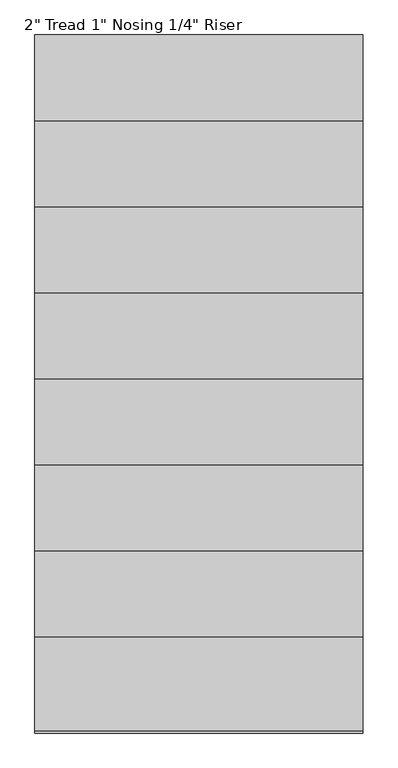
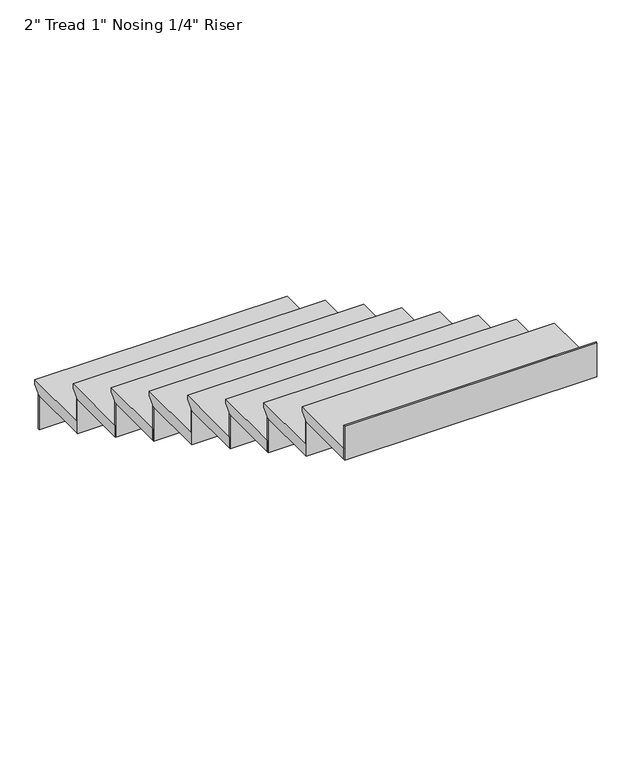
"""IFC4 building model written with IfcOpenShell, lengths in millimetres: stair flight geometry."""

from ifc_helpers import new_model, si_unit, frame, origin, place, context, project, spatial, polyline, outline, extrude, source, transform, mapped, element, save


def stair_flight_8fbc4922(model_context):
    return source(origin(), model_context, "Body", "SweptSolid", [
        extrude(outline(polyline([(-2204.7834702, 4876.8), (-1899.9834702, 4876.8), (-1899.9834702, 4857.75), (-1925.3834702, 4832.35), (-1925.3834702, 4826.0), (-2204.7834702, 4826.0), (-2204.7834702, 4876.8)])), frame((2385.53354, 0.0, 0.0), z_axis=(1.0, 0.0, 0.0), x_axis=(0.0, 1.0, 0.0)), (0.0, 0.0, 1.0), 1066.8),
        extrude(outline(polyline([(2385.53354, -1931.7334702), (2385.53354, -1925.3834702), (3452.33354, -1925.3834702), (3452.33354, -1931.7334702), (2385.53354, -1931.7334702)])), frame((0.0, 0.0, 4673.6), z_axis=(0.0, 0.0, 1.0), x_axis=(1.0, 0.0, 0.0)), (0.0, 0.0, 1.0), 152.4),
        extrude(outline(polyline([(2385.53354, -2211.1334702), (2385.53354, -2204.7834702), (3452.33354, -2204.7834702), (3452.33354, -2211.1334702), (2385.53354, -2211.1334702)])), frame((0.0, 0.0, 4826.0), z_axis=(0.0, 0.0, 1.0), x_axis=(1.0, 0.0, 0.0)), (0.0, 0.0, 1.0), 152.4),
        extrude(outline(polyline([(-2484.1834702, 5029.2), (-2179.3834702, 5029.2), (-2179.3834702, 5010.15), (-2204.7834702, 4984.75), (-2204.7834702, 4978.4), (-2484.1834702, 4978.4), (-2484.1834702, 5029.2)])), frame((2385.53354, 0.0, 0.0), z_axis=(1.0, 0.0, 0.0), x_axis=(0.0, 1.0, 0.0)), (0.0, 0.0, 1.0), 1066.8),
        extrude(outline(polyline([(2385.53354, -2490.5334702), (2385.53354, -2484.1834702), (3452.33354, -2484.1834702), (3452.33354, -2490.5334702), (2385.53354, -2490.5334702)])), frame((0.0, 0.0, 4978.4), z_axis=(0.0, 0.0, 1.0), x_axis=(1.0, 0.0, 0.0)), (0.0, 0.0, 1.0), 152.4),
        extrude(outline(polyline([(-2763.5834702, 5181.6), (-2458.7834702, 5181.6), (-2458.7834702, 5162.55), (-2484.1834702, 5137.15), (-2484.1834702, 5130.8), (-2763.5834702, 5130.8), (-2763.5834702, 5181.6)])), frame((2385.53354, 0.0, 0.0), z_axis=(1.0, 0.0, 0.0), x_axis=(0.0, 1.0, 0.0)), (0.0, 0.0, 1.0), 1066.8),
        extrude(outline(polyline([(2385.53354, -2769.9334702), (2385.53354, -2763.5834702), (3452.33354, -2763.5834702), (3452.33354, -2769.9334702), (2385.53354, -2769.9334702)])), frame((0.0, 0.0, 5130.8), z_axis=(0.0, 0.0, 1.0), x_axis=(1.0, 0.0, 0.0)), (0.0, 0.0, 1.0), 152.4),
        extrude(outline(polyline([(-3042.9834702, 5334.0), (-2738.1834702, 5334.0), (-2738.1834702, 5314.95), (-2763.5834702, 5289.55), (-2763.5834702, 5283.2), (-3042.9834702, 5283.2), (-3042.9834702, 5334.0)])), frame((2385.53354, 0.0, 0.0), z_axis=(1.0, 0.0, 0.0), x_axis=(0.0, 1.0, 0.0)), (0.0, 0.0, 1.0), 1066.8),
        extrude(outline(polyline([(2385.53354, -3049.3334702), (2385.53354, -3042.9834702), (3452.33354, -3042.9834702), (3452.33354, -3049.3334702), (2385.53354, -3049.3334702)])), frame((0.0, 0.0, 5283.2), z_axis=(0.0, 0.0, 1.0), x_axis=(1.0, 0.0, 0.0)), (0.0, 0.0, 1.0), 152.4),
        extrude(outline(polyline([(-3322.3834702, 5486.4), (-3017.5834702, 5486.4), (-3017.5834702, 5467.35), (-3042.9834702, 5441.95), (-3042.9834702, 5435.6), (-3322.3834702, 5435.6), (-3322.3834702, 5486.4)])), frame((2385.53354, 0.0, 0.0), z_axis=(1.0, 0.0, 0.0), x_axis=(0.0, 1.0, 0.0)), (0.0, 0.0, 1.0), 1066.8),
        extrude(outline(polyline([(2385.53354, -3328.7334702), (2385.53354, -3322.3834702), (3452.33354, -3322.3834702), (3452.33354, -3328.7334702), (2385.53354, -3328.7334702)])), frame((0.0, 0.0, 5435.6), z_axis=(0.0, 0.0, 1.0), x_axis=(1.0, 0.0, 0.0)), (0.0, 0.0, 1.0), 152.4),
        extrude(outline(polyline([(-3601.7834702, 5638.8), (-3296.9834702, 5638.8), (-3296.9834702, 5619.75), (-3322.3834702, 5594.35), (-3322.3834702, 5588.0), (-3601.7834702, 5588.0), (-3601.7834702, 5638.8)])), frame((2385.53354, 0.0, 0.0), z_axis=(1.0, 0.0, 0.0), x_axis=(0.0, 1.0, 0.0)), (0.0, 0.0, 1.0), 1066.8),
        extrude(outline(polyline([(2385.53354, -3608.1334702), (2385.53354, -3601.7834702), (3452.33354, -3601.7834702), (3452.33354, -3608.1334702), (2385.53354, -3608.1334702)])), frame((0.0, 0.0, 5588.0), z_axis=(0.0, 0.0, 1.0), x_axis=(1.0, 0.0, 0.0)), (0.0, 0.0, 1.0), 152.4),
        extrude(outline(polyline([(-3881.1834702, 5791.2), (-3576.3834702, 5791.2), (-3576.3834702, 5772.15), (-3601.7834702, 5746.75), (-3601.7834702, 5740.4), (-3881.1834702, 5740.4), (-3881.1834702, 5791.2)])), frame((2385.53354, 0.0, 0.0), z_axis=(1.0, 0.0, 0.0), x_axis=(0.0, 1.0, 0.0)), (0.0, 0.0, 1.0), 1066.8),
        extrude(outline(polyline([(2385.53354, -3887.5334702), (2385.53354, -3881.1834702), (3452.33354, -3881.1834702), (3452.33354, -3887.5334702), (2385.53354, -3887.5334702)])), frame((0.0, 0.0, 5740.4), z_axis=(0.0, 0.0, 1.0), x_axis=(1.0, 0.0, 0.0)), (0.0, 0.0, 1.0), 152.4),
        extrude(outline(polyline([(2385.53354, -4166.9334702), (2385.53354, -4160.5834702), (3452.33354, -4160.5834702), (3452.33354, -4166.9334702), (2385.53354, -4166.9334702)])), frame((0.0, 0.0, 5892.8), z_axis=(0.0, 0.0, 1.0), x_axis=(1.0, 0.0, 0.0)), (0.0, 0.0, 1.0), 152.4),
        extrude(outline(polyline([(-4160.5834702, 5943.6), (-3855.7834702, 5943.6), (-3855.7834702, 5924.55), (-3881.1834702, 5899.15), (-3881.1834702, 5892.8), (-4160.5834702, 5892.8), (-4160.5834702, 5943.6)])), frame((2385.53354, 0.0, 0.0), z_axis=(1.0, 0.0, 0.0), x_axis=(0.0, 1.0, 0.0)), (0.0, 0.0, 1.0), 1066.8),
    ])


if __name__ == "__main__":
    model = new_model("IFC4")
    model_context = context("Model", 3, world=origin())
    ifc_project = project(units=[si_unit("LENGTHUNIT", "METRE", prefix="MILLI")], contexts=[model_context])
    site = spatial("IfcSite", under=ifc_project)
    building = spatial("IfcBuilding", under=site)
    placement = place(None, origin())
    stair_flight_shape = stair_flight_8fbc4922(model_context)
    element("IfcStairFlight", 1, ObjectType="2\" Tread 1\" Nosing 1/4\" Riser", at=placement, inside=building, context=model_context, shape_type="MappedRepresentation", body=[
        mapped(stair_flight_shape, transform((0.0, 0.0, 0.0), x_axis=(1.0, 0.0, 0.0), y_axis=(0.0, 1.0, 0.0), z_axis=(0.0, 0.0, 1.0))),
    ])
    save(model, "model.ifc")
